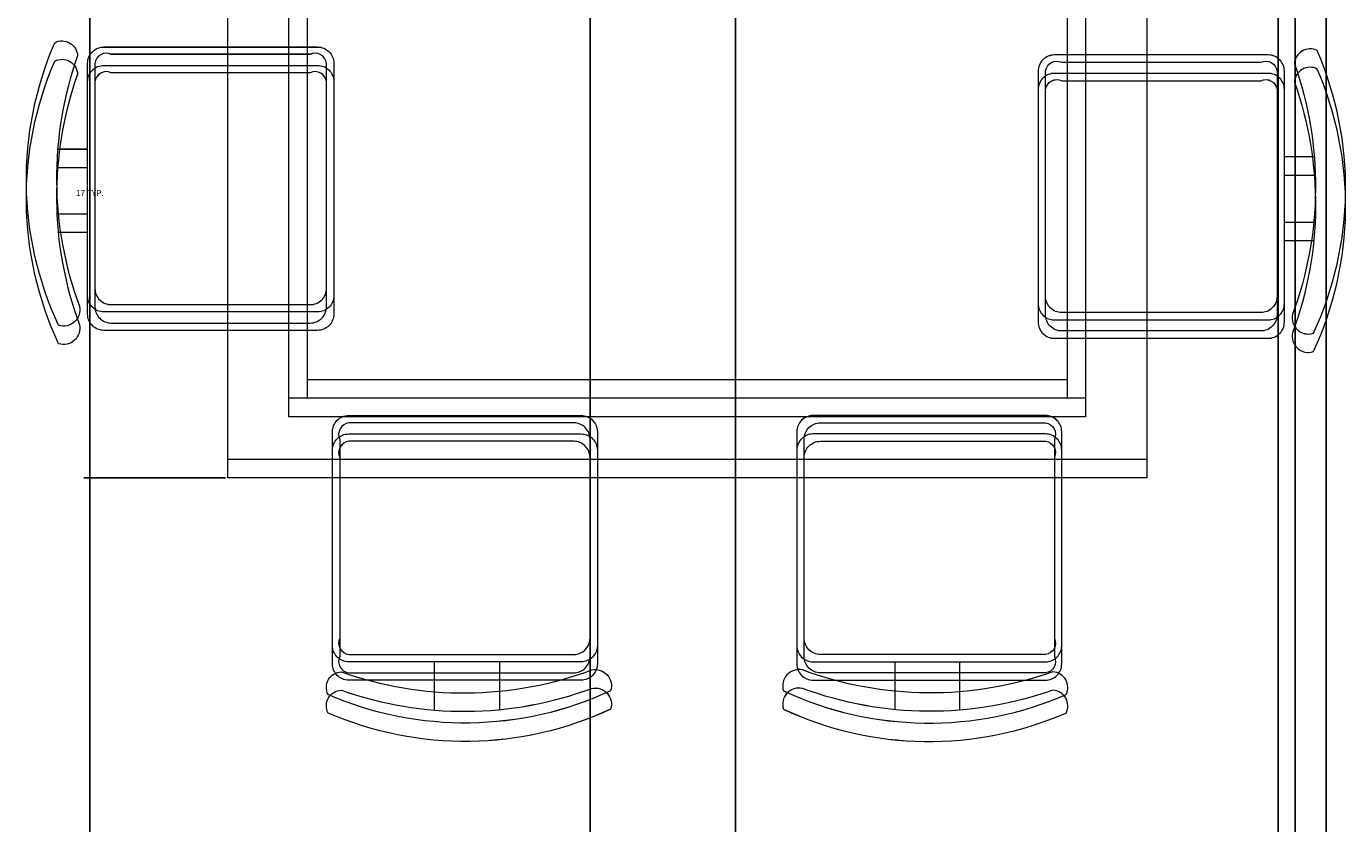
# Model space of a CAD drawing. Units: inches. Extents: x 2063 to 2617, y 1299 to 2210.
# Tile 10 of 22: x 2243 to 2282, y 1901 to 1925. Entities that reach past the tile are written whole.
import ezdxf

# ---------------------------------------------------------------- set-up
doc = ezdxf.new("R2010")
doc.units = ezdxf.units.IN
doc.layers.add('A-ANNO-DIMS', color=2, linetype='Continuous', lineweight=18)
doc.layers.add('A-FURN', color=8, linetype='Continuous', lineweight=18)
doc.styles.get("Standard").update_dxf_attribs({"font": 'arial.ttf'})
doc.dimstyles.get("Standard").update_dxf_attribs({"dimtxt": 0.18, "dimasz": 0.18, "dimexe": 0.18, "dimexo": 0.0625, "dimgap": 0.09, "dimtad": 0, "dimtih": 1, "dimtoh": 1, "dimdec": 4, "dimzin": 0, "dimdsep": 46, "dimtxsty": 'Standard', "dimcen": 0.09, "dimadec": 0, "dimazin": 0, "dimtfac": 1, "dimtdec": 4, "dimtofl": 0, "dimtmove": 0, "dimatfit": 3, "dimfxl": 1, "dimtolj": 1, "dimtzin": 0, "dimarcsym": 0})

# ---------------------------------------------------------------- blocks, each defined once
blk = doc.blocks.new('TABLE-DINING')
for points in [[(0, 17.017), (27.446, 17.017), (27.446, 0.549), (0, 0.549)], [(0, 17.017), (27.446, 17.017), (27.446, 0.549), (0, 0.549)], [(0, 17.016), (27.446, 17.016), (27.446, 0.549), (0, 0.549)], [(0, 17.016), (27.446, 17.016), (27.446, 0.549), (0, 0.549)], [(0, 16.468), (27.446, 16.468), (27.446, 0), (0, 0)], [(0, 16.468), (27.446, 16.468), (27.446, 0), (0, 0)], [(0, 16.467), (27.446, 16.467), (27.446, 0), (0, 0)], [(0, 16.467), (27.446, 16.467), (27.446, 0), (0, 0)], [(1.83, 15.187), (25.616, 15.187), (25.616, 2.379), (1.83, 2.379)], [(1.83, 15.187), (25.616, 15.187), (25.616, 2.379), (1.83, 2.379)], [(1.83, 15.187), (25.616, 15.187), (25.616, 2.379), (1.83, 2.379)], [(1.83, 15.187), (25.616, 15.187), (25.616, 2.379), (1.83, 2.379)], [(1.83, 14.638), (25.616, 14.638), (25.616, 1.83), (1.83, 1.83)], [(1.83, 14.638), (25.616, 14.638), (25.616, 1.83), (1.83, 1.83)], [(1.83, 14.638), (25.616, 14.638), (25.616, 1.83), (1.83, 1.83)], [(1.83, 14.638), (25.616, 14.638), (25.616, 1.83), (1.83, 1.83)], [(2.379, 14.638), (25.067, 14.638), (25.067, 2.928), (2.379, 2.928)], [(2.379, 14.638), (25.067, 14.638), (25.067, 2.927), (2.379, 2.927)], [(2.379, 14.638), (25.067, 14.638), (25.067, 2.928), (2.379, 2.928)], [(2.379, 14.638), (25.067, 14.638), (25.067, 2.927), (2.379, 2.927)], [(2.379, 14.089), (25.067, 14.089), (25.067, 2.379), (2.379, 2.379)], [(2.379, 14.089), (25.067, 14.089), (25.067, 2.379), (2.379, 2.379)], [(2.379, 14.089), (25.067, 14.089), (25.067, 2.379), (2.379, 2.379)], [(2.379, 14.089), (25.067, 14.089), (25.067, 2.379), (2.379, 2.379)]]:
    blk.add_lwpolyline(points, close=True)
blk = doc.blocks.new('*D26')
at = {"layer": 'A-ANNO-DIMS', "color": 0, "lineweight": -2, "transparency": 16777216}
for p, q in [((2248.921, 1928.735), (2244.686, 1928.735)), ((2244.866, 1928.555), (2244.866, 1920.407)), ((2244.866, 1911.898), (2244.866, 1920.046)), ((2248.921, 1911.718), (2244.686, 1911.718))]:
    blk.add_line(p, q, dxfattribs=at)
at = {"layer": 'A-ANNO-DIMS', "color": 0, "transparency": 16777216}
for points in [[(2244.836, 1928.555), (2244.896, 1928.555), (2244.866, 1928.735)], [(2244.836, 1911.898), (2244.896, 1911.898), (2244.866, 1911.718)]]:
    blk.add_solid(points, dxfattribs=at)
at = {"layer": 'Defpoints', "color": 0, "transparency": 16777216}
for p in [(2244.866, 1928.735), (2248.983, 1928.735), (2248.983, 1911.718)]:
    blk.add_point(p, dxfattribs=at)
at = {"layer": 'A-ANNO-DIMS', "color": 0, "transparency": 16777216, "insert": (2244.866, 1920.226), "char_height": 0.18, "attachment_point": 5}
blk.add_mtext('\\A1;17 TYP.', dxfattribs=at)
blk = doc.blocks.new('*D50')
at = {"layer": 'A-ANNO-DIMS', "color": 0, "lineweight": -2, "transparency": 16777216}
for p, q in [((2264.144, 2124.25), (2264.144, 1317.702)), ((2280.348, 2124.25), (2280.348, 1317.702)), ((2264.324, 1317.882), (2271.791, 1317.882)), ((2280.168, 1317.882), (2272.701, 1317.882))]:
    blk.add_line(p, q, dxfattribs=at)
at = {"layer": 'A-ANNO-DIMS', "color": 0, "transparency": 16777216}
for points in [[(2264.324, 1317.912), (2264.324, 1317.852), (2264.144, 1317.882)], [(2280.168, 1317.912), (2280.168, 1317.852), (2280.348, 1317.882)]]:
    blk.add_solid(points, dxfattribs=at)
at = {"layer": 'Defpoints', "color": 0, "transparency": 16777216}
for p in [(2264.144, 2124.312), (2280.348, 2124.312), (2280.348, 1317.882)]:
    blk.add_point(p, dxfattribs=at)
at = {"layer": 'A-ANNO-DIMS', "color": 0, "transparency": 16777216, "insert": (2272.246, 1317.882), "char_height": 0.18, "attachment_point": 5}
blk.add_mtext('\\A1;16.204', dxfattribs=at)
blk = doc.blocks.new('*D62')
at = {"layer": 'A-ANNO-DIMS', "color": 0, "lineweight": -2, "transparency": 16777216}
for p, q in [((2259.809, 1437.875), (2259.809, 2170.742)), ((2281.788, 1437.875), (2281.788, 2170.742)), ((2259.989, 2170.562), (2270.403, 2170.562)), ((2281.608, 2170.562), (2271.194, 2170.562))]:
    blk.add_line(p, q, dxfattribs=at)
at = {"layer": 'A-ANNO-DIMS', "color": 0, "transparency": 16777216}
for points in [[(2259.989, 2170.592), (2259.989, 2170.532), (2259.809, 2170.562)], [(2281.608, 2170.592), (2281.608, 2170.532), (2281.788, 2170.562)]]:
    blk.add_solid(points, dxfattribs=at)
at = {"layer": 'Defpoints', "color": 0, "transparency": 16777216}
for p in [(2281.788, 2170.562), (2259.809, 1437.812), (2281.788, 1437.812)]:
    blk.add_point(p, dxfattribs=at)
at = {"layer": 'A-ANNO-DIMS', "color": 0, "transparency": 16777216, "insert": (2270.798, 2170.562), "char_height": 0.18, "attachment_point": 5}
blk.add_mtext('\\A1;21.98', dxfattribs=at)
blk = doc.blocks.new('*D63')
at = {"layer": 'A-ANNO-DIMS', "color": 0, "lineweight": -2, "transparency": 16777216}
for p, q in [((2244.867, 1562.375), (2244.867, 2170.742)), ((2280.862, 1562.375), (2280.862, 2170.742)), ((2245.047, 2170.562), (2262.4, 2170.562)), ((2280.682, 2170.562), (2263.329, 2170.562))]:
    blk.add_line(p, q, dxfattribs=at)
at = {"layer": 'A-ANNO-DIMS', "color": 0, "transparency": 16777216}
for points in [[(2245.047, 2170.592), (2245.047, 2170.532), (2244.867, 2170.562)], [(2280.682, 2170.592), (2280.682, 2170.532), (2280.862, 2170.562)]]:
    blk.add_solid(points, dxfattribs=at)
at = {"layer": 'Defpoints', "color": 0, "transparency": 16777216}
for p in [(2280.862, 2170.562), (2244.867, 1562.312), (2280.862, 1562.312)]:
    blk.add_point(p, dxfattribs=at)
at = {"layer": 'A-ANNO-DIMS', "color": 0, "transparency": 16777216, "insert": (2262.865, 2170.562), "char_height": 0.18, "attachment_point": 5}
blk.add_mtext('\\A1;35.995', dxfattribs=at)

msp = doc.modelspace()

# ---------------------------------------------------------------- linework, layer by layer
at = {"layer": 'A-FURN'}
for points in [[(2244.5572, 1916.8435, -0.5783921), (2243.9345, 1916.2772, -0.2145244), (2243.8212, 1924.7154, -0.552014), (2244.5006, 1924.319, 0.1758094), (2244.5572, 1916.8435)], [(2244.5572, 1916.8435, -0.5783921), (2243.9345, 1916.2772, -0.2145244), (2243.8212, 1924.7154, -0.552014), (2244.5006, 1924.319, 0.1758094), (2244.5572, 1916.8435)], [(2244.5572, 1916.8433, -0.5783921), (2243.9345, 1916.2769, -0.2145244), (2243.8213, 1924.7151, -0.552014), (2244.5006, 1924.3187, 0.1758094), (2244.5572, 1916.8432)], [(2244.5572, 1916.8433, -0.5783921), (2243.9345, 1916.2769, -0.2145244), (2243.8213, 1924.7151, -0.552014), (2244.5006, 1924.3187, 0.1758094), (2244.5572, 1916.8432)], [(2244.8006, 1924.1006, -0.4142136), (2245.2861, 1924.5862), (2251.6673, 1924.5862, -0.4142136), (2252.1528, 1924.1006), (2252.1528, 1917.1607, -0.4142136), (2251.6673, 1916.6752), (2245.2861, 1916.6752, -0.4142136), (2244.8006, 1917.1607), (2244.8006, 1924.1006)], [(2244.8006, 1924.1006, -0.4142136), (2245.2861, 1924.5862), (2251.6673, 1924.5862, -0.4142136), (2252.1528, 1924.1006), (2252.1528, 1917.1607, -0.4142136), (2251.6673, 1916.6752), (2245.2861, 1916.6752, -0.4142136), (2244.8006, 1917.1607), (2244.8006, 1924.1006)], [(2244.8006, 1924.1003, -0.4142136), (2245.2861, 1924.5859), (2251.6673, 1924.5859, -0.4142136), (2252.1528, 1924.1003), (2252.1528, 1917.1604, -0.4142136), (2251.6673, 1916.6749), (2245.2861, 1916.6749, -0.4142136), (2244.8006, 1917.1604), (2244.8006, 1924.1003)], [(2244.8006, 1924.1003, -0.4142136), (2245.2861, 1924.5859), (2251.6673, 1924.5859, -0.4142136), (2252.1528, 1924.1003), (2252.1528, 1917.1604, -0.4142136), (2251.6673, 1916.6749), (2245.2861, 1916.6749, -0.4142136), (2244.8006, 1917.1604), (2244.8006, 1924.1003)], [(2280.8381, 1924.0813, -0.1758092), (2280.7815, 1916.6059, 0.5783921), (2281.4042, 1916.0395, 0.2145244), (2281.5174, 1924.4777, 0.552014), (2280.8381, 1924.0813, -0.065079)], [(2280.8381, 1924.0813, -0.1758092), (2280.7815, 1916.6059, 0.5783921), (2281.4042, 1916.0395, 0.2145244), (2281.5174, 1924.4777, 0.552014), (2280.8381, 1924.0813, -0.065079)], [(2280.8381, 1924.081, -0.1758092), (2280.7815, 1916.6056, 0.5783921), (2281.4042, 1916.0392, 0.2145244), (2281.5174, 1924.4774, 0.552014), (2280.8381, 1924.081, -0.065079)], [(2280.8381, 1924.081, -0.1758092), (2280.7815, 1916.6056, 0.5783921), (2281.4042, 1916.0392, 0.2145244), (2281.5174, 1924.4774, 0.552014), (2280.8381, 1924.081, -0.065079)], [(2244.5572, 1916.2946, -0.5783921), (2243.9345, 1915.7283, -0.2145244), (2243.8212, 1924.1665, -0.552014), (2244.5006, 1923.7701, 0.1758094), (2244.5572, 1916.2946)], [(2244.5572, 1916.2946, -0.5783921), (2243.9345, 1915.7283, -0.2145244), (2243.8212, 1924.1665, -0.552014), (2244.5006, 1923.7701, 0.1758094), (2244.5572, 1916.2946)], [(2244.5572, 1916.2943, -0.5783921), (2243.9345, 1915.728, -0.2145244), (2243.8213, 1924.1662, -0.552014), (2244.5006, 1923.7698, 0.1758094), (2244.5572, 1916.2943)], [(2244.5572, 1916.2943, -0.5783921), (2243.9345, 1915.728, -0.2145244), (2243.8213, 1924.1662, -0.552014), (2244.5006, 1923.7698, 0.1758094), (2244.5572, 1916.2943)], [(2280.5381, 1923.863, 0.4142136), (2280.0525, 1924.3485), (2273.6714, 1924.3485, 0.4142136), (2273.1859, 1923.863), (2273.1859, 1916.923, 0.4142136), (2273.6714, 1916.4375), (2280.0525, 1916.4375, 0.4142136), (2280.5381, 1916.923), (2280.5381, 1923.863)], [(2280.5381, 1923.863, 0.4142136), (2280.0525, 1924.3485), (2273.6714, 1924.3485, 0.4142136), (2273.1859, 1923.863), (2273.1859, 1916.923, 0.4142136), (2273.6714, 1916.4375), (2280.0525, 1916.4375, 0.4142136), (2280.5381, 1916.923), (2280.5381, 1923.863)], [(2280.5381, 1923.8627, 0.4142136), (2280.0526, 1924.3482), (2273.6714, 1924.3482, 0.4142136), (2273.1859, 1923.8627), (2273.1859, 1916.9227, 0.4142136), (2273.6714, 1916.4372), (2280.0526, 1916.4372, 0.4142136), (2280.5381, 1916.9227), (2280.5381, 1923.8627)], [(2280.5381, 1923.8627, 0.4142136), (2280.0526, 1924.3482), (2273.6714, 1924.3482, 0.4142136), (2273.1859, 1923.8627), (2273.1859, 1916.9227, 0.4142136), (2273.6714, 1916.4372), (2280.0526, 1916.4372, 0.4142136), (2280.5381, 1916.9227), (2280.5381, 1923.8627)], [(2244.8006, 1923.5517, -0.4142136), (2245.2861, 1924.0372), (2251.6673, 1924.0372, -0.4142136), (2252.1528, 1923.5517), (2252.1528, 1916.6118, -0.4142136), (2251.6673, 1916.1262), (2245.2861, 1916.1262, -0.4142136), (2244.8006, 1916.6118), (2244.8006, 1923.5517)], [(2244.8006, 1923.5517, -0.4142136), (2245.2861, 1924.0372), (2251.6673, 1924.0372, -0.4142136), (2252.1528, 1923.5517), (2252.1528, 1916.6118, -0.4142136), (2251.6673, 1916.1262), (2245.2861, 1916.1262, -0.4142136), (2244.8006, 1916.6118), (2244.8006, 1923.5517)], [(2244.8006, 1923.5514, -0.4142136), (2245.2861, 1924.037), (2251.6673, 1924.037, -0.4142136), (2252.1528, 1923.5514), (2252.1528, 1916.6115, -0.4142136), (2251.6673, 1916.126), (2245.2861, 1916.126, -0.4142136), (2244.8006, 1916.6115), (2244.8006, 1923.5514)], [(2244.8006, 1923.5514, -0.4142136), (2245.2861, 1924.037), (2251.6673, 1924.037, -0.4142136), (2252.1528, 1923.5514), (2252.1528, 1916.6115, -0.4142136), (2251.6673, 1916.126), (2245.2861, 1916.126, -0.4142136), (2244.8006, 1916.6115), (2244.8006, 1923.5514)], [(2280.5381, 1923.314, 0.4142136), (2280.0525, 1923.7996), (2273.6714, 1923.7996, 0.4142136), (2273.1859, 1923.314), (2273.1859, 1916.3741, 0.4142136), (2273.6714, 1915.8886), (2280.0525, 1915.8886, 0.4142136), (2280.5381, 1916.3741), (2280.5381, 1923.314)], [(2280.5381, 1923.314, 0.4142136), (2280.0525, 1923.7996), (2273.6714, 1923.7996, 0.4142136), (2273.1859, 1923.314), (2273.1859, 1916.3741, 0.4142136), (2273.6714, 1915.8886), (2280.0525, 1915.8886, 0.4142136), (2280.5381, 1916.3741), (2280.5381, 1923.314)], [(2280.5381, 1923.3138, 0.4142136), (2280.0526, 1923.7993), (2273.6714, 1923.7993, 0.4142136), (2273.1859, 1923.3138), (2273.1859, 1916.3738, 0.4142136), (2273.6714, 1915.8883), (2280.0526, 1915.8883, 0.4142136), (2280.5381, 1916.3738), (2280.5381, 1923.3138)], [(2280.5381, 1923.3138, 0.4142136), (2280.0526, 1923.7993), (2273.6714, 1923.7993, 0.4142136), (2273.1859, 1923.3138), (2273.1859, 1916.3738, 0.4142136), (2273.6714, 1915.8883), (2280.0526, 1915.8883, 0.4142136), (2280.5381, 1916.3738), (2280.5381, 1923.3138)], [(2280.8381, 1923.5324, -0.1758092), (2280.7815, 1916.0569, 0.5783921), (2281.4042, 1915.4906, 0.2145244), (2281.5174, 1923.9288, 0.552014), (2280.8381, 1923.5324, -0.065079)], [(2280.8381, 1923.5324, -0.1758092), (2280.7815, 1916.0569, 0.5783921), (2281.4042, 1915.4906, 0.2145244), (2281.5174, 1923.9288, 0.552014), (2280.8381, 1923.5324, -0.065079)], [(2280.8381, 1923.5321, -0.1758092), (2280.7815, 1916.0567, 0.5783921), (2281.4042, 1915.4903, 0.2145244), (2281.5174, 1923.9285, 0.552014), (2280.8381, 1923.5321, -0.065079)], [(2280.8381, 1923.5321, -0.1758092), (2280.7815, 1916.0567, 0.5783921), (2281.4042, 1915.4903, 0.2145244), (2281.5174, 1923.9285, 0.552014), (2280.8381, 1923.5321, -0.065079)], [(2244.8006, 1919.5983), (2243.9229, 1919.5983, 0.0647586)], [(2244.8006, 1919.5983), (2243.9229, 1919.5983, 0.0647586)], [(2244.8006, 1919.5981), (2243.9229, 1919.5981, 0.0647586)], [(2244.8006, 1919.5981), (2243.9229, 1919.5981, 0.0647586)], [(2280.5381, 1919.3607), (2281.4158, 1919.3607, -0.0647586)], [(2280.5381, 1919.3607), (2281.4158, 1919.3607, -0.0647586)], [(2280.5381, 1919.3604), (2281.4158, 1919.3604, -0.0647586)], [(2280.5381, 1919.3604), (2281.4158, 1919.3604, -0.0647586)], [(2244.8006, 1919.0494), (2243.9229, 1919.0494, 0.0647586)], [(2244.8006, 1919.0494), (2243.9229, 1919.0494, 0.0647586)], [(2244.8006, 1919.0491), (2243.9229, 1919.0491, 0.0647586)], [(2244.8006, 1919.0491), (2243.9229, 1919.0491, 0.0647586)], [(2280.5381, 1918.8118), (2281.4158, 1918.8118, -0.0647586)], [(2280.5381, 1918.8118), (2281.4158, 1918.8118, -0.0647586)], [(2280.5381, 1918.8115), (2281.4158, 1918.8115, -0.0647586)], [(2280.5381, 1918.8115), (2281.4158, 1918.8115, -0.0647586)], [(2259.5362, 1906.2298), (2252.5963, 1906.2298, -0.4142136), (2252.1107, 1906.7153), (2252.1107, 1913.0965, -0.4142136), (2252.5963, 1913.582), (2259.5362, 1913.582, -0.4142136), (2260.0217, 1913.0965), (2260.0217, 1906.7153, -0.4142136), (2259.5362, 1906.2298)], [(2259.5362, 1906.2298), (2252.5963, 1906.2298, -0.4142136), (2252.1107, 1906.7153), (2252.1107, 1913.0965, -0.4142136), (2252.5963, 1913.582), (2259.5362, 1913.582, -0.4142136), (2260.0217, 1913.0965), (2260.0217, 1906.7153, -0.4142136), (2259.5362, 1906.2298)], [(2259.5362, 1906.2295), (2252.5963, 1906.2295, -0.4142136), (2252.1108, 1906.715), (2252.1108, 1913.0962, -0.4142136), (2252.5963, 1913.5817), (2259.5362, 1913.5817, -0.4142136), (2260.0218, 1913.0962), (2260.0218, 1906.715, -0.4142136), (2259.5362, 1906.2295)], [(2259.5362, 1906.2295), (2252.5963, 1906.2295, -0.4142136), (2252.1108, 1906.715), (2252.1108, 1913.0962, -0.4142136), (2252.5963, 1913.5817), (2259.5362, 1913.5817, -0.4142136), (2260.0218, 1913.0962), (2260.0218, 1906.715, -0.4142136), (2259.5362, 1906.2295)], [(2273.4038, 1906.2298, 0.4142136), (2273.8893, 1906.7153), (2273.8893, 1913.0965, 0.4142136), (2273.4038, 1913.582), (2266.4639, 1913.582, 0.4142136), (2265.9783, 1913.0965), (2265.9783, 1906.7153, 0.4142136), (2266.4639, 1906.2298), (2273.4038, 1906.2298)], [(2273.4038, 1906.2298, 0.4142136), (2273.8893, 1906.7153), (2273.8893, 1913.0965, 0.4142136), (2273.4038, 1913.582), (2266.4639, 1913.582, 0.4142136), (2265.9783, 1913.0965), (2265.9783, 1906.7153, 0.4142136), (2266.4639, 1906.2298), (2273.4038, 1906.2298)], [(2273.4038, 1906.2295, 0.4142136), (2273.8893, 1906.715), (2273.8893, 1913.0962, 0.4142136), (2273.4038, 1913.5817), (2266.4639, 1913.5817, 0.4142136), (2265.9784, 1913.0962), (2265.9784, 1906.715, 0.4142136), (2266.4639, 1906.2295), (2273.4038, 1906.2295)], [(2273.4038, 1906.2295, 0.4142136), (2273.8893, 1906.715), (2273.8893, 1913.0962, 0.4142136), (2273.4038, 1913.5817), (2266.4639, 1913.5817, 0.4142136), (2265.9784, 1913.0962), (2265.9784, 1906.715, 0.4142136), (2266.4639, 1906.2295), (2273.4038, 1906.2295)], [(2259.5362, 1905.6809), (2252.5963, 1905.6809, -0.4142136), (2252.1107, 1906.1664), (2252.1107, 1912.5476, -0.4142136), (2252.5963, 1913.0331), (2259.5362, 1913.0331, -0.4142136), (2260.0217, 1912.5476), (2260.0217, 1906.1664, -0.4142136), (2259.5362, 1905.6809)], [(2259.5362, 1905.6809), (2252.5963, 1905.6809, -0.4142136), (2252.1107, 1906.1664), (2252.1107, 1912.5476, -0.4142136), (2252.5963, 1913.0331), (2259.5362, 1913.0331, -0.4142136), (2260.0217, 1912.5476), (2260.0217, 1906.1664, -0.4142136), (2259.5362, 1905.6809)], [(2259.5362, 1905.6806), (2252.5963, 1905.6806, -0.4142136), (2252.1108, 1906.1661), (2252.1108, 1912.5473, -0.4142136), (2252.5963, 1913.0328), (2259.5362, 1913.0328, -0.4142136), (2260.0218, 1912.5473), (2260.0218, 1906.1661, -0.4142136), (2259.5362, 1905.6806)], [(2259.5362, 1905.6806), (2252.5963, 1905.6806, -0.4142136), (2252.1108, 1906.1661), (2252.1108, 1912.5473, -0.4142136), (2252.5963, 1913.0328), (2259.5362, 1913.0328, -0.4142136), (2260.0218, 1912.5473), (2260.0218, 1906.1661, -0.4142136), (2259.5362, 1905.6806)], [(2273.4038, 1905.6809, 0.4142136), (2273.8893, 1906.1664), (2273.8893, 1912.5476, 0.4142136), (2273.4038, 1913.0331), (2266.4639, 1913.0331, 0.4142136), (2265.9783, 1912.5476), (2265.9783, 1906.1664, 0.4142136), (2266.4639, 1905.6809), (2273.4038, 1905.6809)], [(2273.4038, 1905.6809, 0.4142136), (2273.8893, 1906.1664), (2273.8893, 1912.5476, 0.4142136), (2273.4038, 1913.0331), (2266.4639, 1913.0331, 0.4142136), (2265.9783, 1912.5476), (2265.9783, 1906.1664, 0.4142136), (2266.4639, 1905.6809), (2273.4038, 1905.6809)], [(2273.4038, 1905.6806, 0.4142136), (2273.8893, 1906.1661), (2273.8893, 1912.5473, 0.4142136), (2273.4038, 1913.0328), (2266.4639, 1913.0328, 0.4142136), (2265.9784, 1912.5473), (2265.9784, 1906.1661, 0.4142136), (2266.4639, 1905.6806), (2273.4038, 1905.6806)], [(2273.4038, 1905.6806, 0.4142136), (2273.8893, 1906.1661), (2273.8893, 1912.5473, 0.4142136), (2273.4038, 1913.0328), (2266.4639, 1913.0328, 0.4142136), (2265.9784, 1912.5473), (2265.9784, 1906.1661, 0.4142136), (2266.4639, 1905.6806), (2273.4038, 1905.6806)], [(2259.8534, 1905.9864, -0.5783921), (2260.4197, 1905.3637, -0.2145244), (2251.9815, 1905.2505, -0.552014), (2252.3779, 1905.9298, 0.1758093), (2259.8534, 1905.9864)], [(2259.8534, 1905.9864, -0.5783921), (2260.4197, 1905.3637, -0.2145244), (2251.9815, 1905.2505, -0.552014), (2252.3779, 1905.9298, 0.1758093), (2259.8534, 1905.9864)], [(2259.8534, 1905.9861, -0.5783921), (2260.4197, 1905.3634, -0.2145244), (2251.9815, 1905.2502, -0.552014), (2252.3779, 1905.9295, 0.1758093), (2259.8534, 1905.9861)], [(2259.8534, 1905.9861, -0.5783921), (2260.4197, 1905.3634, -0.2145244), (2251.9815, 1905.2502, -0.552014), (2252.3779, 1905.9295, 0.1758093), (2259.8534, 1905.9861)], [(2257.0986, 1906.2298), (2257.0986, 1905.3521, 0.0647586)], [(2257.0986, 1906.2298), (2257.0986, 1905.3521, 0.0647586)], [(2257.0986, 1906.2295), (2257.0986, 1905.3518, 0.0647586)], [(2257.0986, 1906.2295), (2257.0986, 1905.3518, 0.0647586)], [(2273.6222, 1905.9298, -0.1758093), (2266.1467, 1905.9864, 0.5783921), (2265.5804, 1905.3637, 0.2145244), (2274.0186, 1905.2505, 0.552014), (2273.6222, 1905.9298, -0.065079)], [(2273.6222, 1905.9298, -0.1758093), (2266.1467, 1905.9864, 0.5783921), (2265.5804, 1905.3637, 0.2145244), (2274.0186, 1905.2505, 0.552014), (2273.6222, 1905.9298, -0.065079)], [(2273.6222, 1905.9295, -0.1758093), (2266.1467, 1905.9861, 0.5783921), (2265.5804, 1905.3634, 0.2145244), (2274.0186, 1905.2502, 0.552014), (2273.6222, 1905.9295, -0.065079)], [(2273.6222, 1905.9295, -0.1758093), (2266.1467, 1905.9861, 0.5783921), (2265.5804, 1905.3634, 0.2145244), (2274.0186, 1905.2502, 0.552014), (2273.6222, 1905.9295, -0.065079)], [(2268.9015, 1906.2298), (2268.9015, 1905.3521, -0.0647586)], [(2268.9015, 1906.2298), (2268.9015, 1905.3521, -0.0647586)], [(2268.9015, 1906.2295), (2268.9015, 1905.3518, -0.0647586)], [(2268.9015, 1906.2295), (2268.9015, 1905.3518, -0.0647586)], [(2257.0986, 1905.6809), (2257.0986, 1904.8032, 0.0647586)], [(2257.0986, 1905.6809), (2257.0986, 1904.8032, 0.0647586)], [(2257.0986, 1905.6806), (2257.0986, 1904.8029, 0.0647586)], [(2257.0986, 1905.6806), (2257.0986, 1904.8029, 0.0647586)], [(2268.9015, 1905.6809), (2268.9015, 1904.8032, -0.0647586)], [(2268.9015, 1905.6809), (2268.9015, 1904.8032, -0.0647586)], [(2268.9015, 1905.6806), (2268.9015, 1904.8029, -0.0647586)], [(2268.9015, 1905.6806), (2268.9015, 1904.8029, -0.0647586)], [(2259.8534, 1905.4375, -0.5783921), (2260.4197, 1904.8148, -0.2145244), (2251.9815, 1904.7015, -0.552014), (2252.3779, 1905.3809, 0.1758093), (2259.8534, 1905.4375)], [(2259.8534, 1905.4375, -0.5783921), (2260.4197, 1904.8148, -0.2145244), (2251.9815, 1904.7015, -0.552014), (2252.3779, 1905.3809, 0.1758093), (2259.8534, 1905.4375)], [(2259.8534, 1905.4372, -0.5783921), (2260.4197, 1904.8145, -0.2145244), (2251.9815, 1904.7012, -0.552014), (2252.3779, 1905.3806, 0.1758093), (2259.8534, 1905.4372)], [(2259.8534, 1905.4372, -0.5783921), (2260.4197, 1904.8145, -0.2145244), (2251.9815, 1904.7012, -0.552014), (2252.3779, 1905.3806, 0.1758093), (2259.8534, 1905.4372)], [(2273.6222, 1905.3809, -0.1758093), (2266.1467, 1905.4375, 0.5783921), (2265.5804, 1904.8148, 0.2145244), (2274.0186, 1904.7015, 0.552014), (2273.6222, 1905.3809, -0.065079)], [(2273.6222, 1905.3809, -0.1758093), (2266.1467, 1905.4375, 0.5783921), (2265.5804, 1904.8148, 0.2145244), (2274.0186, 1904.7015, 0.552014), (2273.6222, 1905.3809, -0.065079)], [(2273.6222, 1905.3806, -0.1758093), (2266.1467, 1905.4372, 0.5783921), (2265.5804, 1904.8145, 0.2145244), (2274.0186, 1904.7012, 0.552014), (2273.6222, 1905.3806, -0.065079)], [(2273.6222, 1905.3806, -0.1758093), (2266.1467, 1905.4372, 0.5783921), (2265.5804, 1904.8145, 0.2145244), (2274.0186, 1904.7012, 0.552014), (2273.6222, 1905.3806, -0.065079)]]:
    msp.add_lwpolyline(points, format="xyb", dxfattribs=at)
for points in [[(2245.0193, 1924.0977), (2245.0193, 1917.3794, 0.4142136), (2245.5049, 1916.8939), (2251.4485, 1916.8939, 0.4142136), (2251.9341, 1917.3794), (2251.9341, 1924.0977, 0.5120695), (2251.4485, 1924.3674), (2245.5049, 1924.3674, 0.5120695)], [(2245.0193, 1924.0977), (2245.0193, 1917.3794, 0.4142136), (2245.5049, 1916.8939), (2251.4485, 1916.8939, 0.4142136), (2251.9341, 1917.3794), (2251.9341, 1924.0977, 0.5120695), (2251.4485, 1924.3674), (2245.5049, 1924.3674, 0.5120695)], [(2245.0193, 1924.0974), (2245.0193, 1917.3791, 0.4142136), (2245.5049, 1916.8936), (2251.4486, 1916.8936, 0.4142136), (2251.9341, 1917.3791), (2251.9341, 1924.0974, 0.5120695), (2251.4486, 1924.3671), (2245.5049, 1924.3671, 0.5120695)], [(2245.0193, 1924.0974), (2245.0193, 1917.3791, 0.4142136), (2245.5049, 1916.8936), (2251.4486, 1916.8936, 0.4142136), (2251.9341, 1917.3791), (2251.9341, 1924.0974, 0.5120695), (2251.4486, 1924.3671), (2245.5049, 1924.3671, 0.5120695)], [(2280.3193, 1923.86), (2280.3193, 1917.1417, -0.4142136), (2279.8338, 1916.6562), (2273.8901, 1916.6562, -0.4142136), (2273.4046, 1917.1417), (2273.4046, 1923.86, -0.5120695), (2273.8901, 1924.1297), (2279.8338, 1924.1297, -0.5120695)], [(2280.3193, 1923.86), (2280.3193, 1917.1417, -0.4142136), (2279.8338, 1916.6562), (2273.8901, 1916.6562, -0.4142136), (2273.4046, 1917.1417), (2273.4046, 1923.86, -0.5120695), (2273.8901, 1924.1297), (2279.8338, 1924.1297, -0.5120695)], [(2280.3193, 1923.8597), (2280.3193, 1917.1415, -0.4142136), (2279.8338, 1916.6559), (2273.8901, 1916.6559, -0.4142136), (2273.4046, 1917.1415), (2273.4046, 1923.8597, -0.5120695), (2273.8901, 1924.1295), (2279.8338, 1924.1295, -0.5120695)], [(2280.3193, 1923.8597), (2280.3193, 1917.1415, -0.4142136), (2279.8338, 1916.6559), (2273.8901, 1916.6559, -0.4142136), (2273.4046, 1917.1415), (2273.4046, 1923.8597, -0.5120695), (2273.8901, 1924.1295), (2279.8338, 1924.1295, -0.5120695)], [(2245.0193, 1923.5488), (2245.0193, 1916.8305, 0.4142136), (2245.5049, 1916.345), (2251.4485, 1916.345, 0.4142136), (2251.9341, 1916.8305), (2251.9341, 1923.5488, 0.5120695), (2251.4485, 1923.8185), (2245.5049, 1923.8185, 0.5120695)], [(2245.0193, 1923.5488), (2245.0193, 1916.8305, 0.4142136), (2245.5049, 1916.345), (2251.4485, 1916.345, 0.4142136), (2251.9341, 1916.8305), (2251.9341, 1923.5488, 0.5120695), (2251.4485, 1923.8185), (2245.5049, 1923.8185, 0.5120695)], [(2245.0193, 1923.5485), (2245.0193, 1916.8302, 0.4142136), (2245.5049, 1916.3447), (2251.4486, 1916.3447, 0.4142136), (2251.9341, 1916.8302), (2251.9341, 1923.5485, 0.5120695), (2251.4486, 1923.8182), (2245.5049, 1923.8182, 0.5120695)], [(2245.0193, 1923.5485), (2245.0193, 1916.8302, 0.4142136), (2245.5049, 1916.3447), (2251.4486, 1916.3447, 0.4142136), (2251.9341, 1916.8302), (2251.9341, 1923.5485, 0.5120695), (2251.4486, 1923.8182), (2245.5049, 1923.8182, 0.5120695)], [(2280.3193, 1923.3111), (2280.3193, 1916.5928, -0.4142136), (2279.8338, 1916.1073), (2273.8901, 1916.1073, -0.4142136), (2273.4046, 1916.5928), (2273.4046, 1923.3111, -0.5120695), (2273.8901, 1923.5808), (2279.8338, 1923.5808, -0.5120695)], [(2280.3193, 1923.3111), (2280.3193, 1916.5928, -0.4142136), (2279.8338, 1916.1073), (2273.8901, 1916.1073, -0.4142136), (2273.4046, 1916.5928), (2273.4046, 1923.3111, -0.5120695), (2273.8901, 1923.5808), (2279.8338, 1923.5808, -0.5120695)], [(2280.3193, 1923.3108), (2280.3193, 1916.5925, -0.4142136), (2279.8338, 1916.107), (2273.8901, 1916.107, -0.4142136), (2273.4046, 1916.5925), (2273.4046, 1923.3108, -0.5120695), (2273.8901, 1923.5805), (2279.8338, 1923.5805, -0.5120695)], [(2280.3193, 1923.3108), (2280.3193, 1916.5925, -0.4142136), (2279.8338, 1916.107), (2273.8901, 1916.107, -0.4142136), (2273.4046, 1916.5925), (2273.4046, 1923.3108, -0.5120695), (2273.8901, 1923.5805), (2279.8338, 1923.5805, -0.5120695)], [(2252.5992, 1906.4485), (2259.3175, 1906.4485, 0.4142136), (2259.803, 1906.9341), (2259.803, 1912.8777, 0.4142136), (2259.3175, 1913.3633), (2252.5992, 1913.3633, 0.5120695), (2252.3295, 1912.8777), (2252.3295, 1906.9341, 0.5120695)], [(2252.5992, 1906.4485), (2259.3175, 1906.4485, 0.4142136), (2259.803, 1906.9341), (2259.803, 1912.8777, 0.4142136), (2259.3175, 1913.3633), (2252.5992, 1913.3633, 0.5120695), (2252.3295, 1912.8777), (2252.3295, 1906.9341, 0.5120695)], [(2252.5992, 1906.4483), (2259.3175, 1906.4483, 0.4142136), (2259.803, 1906.9338), (2259.803, 1912.8775, 0.4142136), (2259.3175, 1913.363), (2252.5992, 1913.363, 0.5120695), (2252.3295, 1912.8775), (2252.3295, 1906.9338, 0.5120695)], [(2252.5992, 1906.4483), (2259.3175, 1906.4483, 0.4142136), (2259.803, 1906.9338), (2259.803, 1912.8775, 0.4142136), (2259.3175, 1913.363), (2252.5992, 1913.363, 0.5120695), (2252.3295, 1912.8775), (2252.3295, 1906.9338, 0.5120695)], [(2273.4009, 1906.4485), (2266.6826, 1906.4485, -0.4142136), (2266.1971, 1906.9341), (2266.1971, 1912.8777, -0.4142136), (2266.6826, 1913.3633), (2273.4009, 1913.3633, -0.5120695), (2273.6706, 1912.8777), (2273.6706, 1906.9341, -0.5120695)], [(2273.4009, 1906.4485), (2266.6826, 1906.4485, -0.4142136), (2266.1971, 1906.9341), (2266.1971, 1912.8777, -0.4142136), (2266.6826, 1913.3633), (2273.4009, 1913.3633, -0.5120695), (2273.6706, 1912.8777), (2273.6706, 1906.9341, -0.5120695)], [(2273.4009, 1906.4483), (2266.6826, 1906.4483, -0.4142136), (2266.1971, 1906.9338), (2266.1971, 1912.8775, -0.4142136), (2266.6826, 1913.363), (2273.4009, 1913.363, -0.5120695), (2273.6706, 1912.8775), (2273.6706, 1906.9338, -0.5120695)], [(2273.4009, 1906.4483), (2266.6826, 1906.4483, -0.4142136), (2266.1971, 1906.9338), (2266.1971, 1912.8775, -0.4142136), (2266.6826, 1913.363), (2273.4009, 1913.363, -0.5120695), (2273.6706, 1912.8775), (2273.6706, 1906.9338, -0.5120695)], [(2252.5992, 1905.8996), (2259.3175, 1905.8996, 0.4142136), (2259.803, 1906.3852), (2259.803, 1912.3288, 0.4142136), (2259.3175, 1912.8144), (2252.5992, 1912.8144, 0.5120695), (2252.3295, 1912.3288), (2252.3295, 1906.3852, 0.5120695)], [(2252.5992, 1905.8996), (2259.3175, 1905.8996, 0.4142136), (2259.803, 1906.3852), (2259.803, 1912.3288, 0.4142136), (2259.3175, 1912.8144), (2252.5992, 1912.8144, 0.5120695), (2252.3295, 1912.3288), (2252.3295, 1906.3852, 0.5120695)], [(2252.5992, 1905.8993), (2259.3175, 1905.8993, 0.4142136), (2259.803, 1906.3849), (2259.803, 1912.3285, 0.4142136), (2259.3175, 1912.8141), (2252.5992, 1912.8141, 0.5120695), (2252.3295, 1912.3285), (2252.3295, 1906.3849, 0.5120695)], [(2252.5992, 1905.8993), (2259.3175, 1905.8993, 0.4142136), (2259.803, 1906.3849), (2259.803, 1912.3285, 0.4142136), (2259.3175, 1912.8141), (2252.5992, 1912.8141, 0.5120695), (2252.3295, 1912.3285), (2252.3295, 1906.3849, 0.5120695)], [(2273.4009, 1905.8996), (2266.6826, 1905.8996, -0.4142136), (2266.1971, 1906.3852), (2266.1971, 1912.3288, -0.4142136), (2266.6826, 1912.8144), (2273.4009, 1912.8144, -0.5120695), (2273.6706, 1912.3288), (2273.6706, 1906.3852, -0.5120695)], [(2273.4009, 1905.8996), (2266.6826, 1905.8996, -0.4142136), (2266.1971, 1906.3852), (2266.1971, 1912.3288, -0.4142136), (2266.6826, 1912.8144), (2273.4009, 1912.8144, -0.5120695), (2273.6706, 1912.3288), (2273.6706, 1906.3852, -0.5120695)], [(2273.4009, 1905.8993), (2266.6826, 1905.8993, -0.4142136), (2266.1971, 1906.3849), (2266.1971, 1912.3285, -0.4142136), (2266.6826, 1912.8141), (2273.4009, 1912.8141, -0.5120695), (2273.6706, 1912.3285), (2273.6706, 1906.3849, -0.5120695)], [(2273.4009, 1905.8993), (2266.6826, 1905.8993, -0.4142136), (2266.1971, 1906.3849), (2266.1971, 1912.3285, -0.4142136), (2266.6826, 1912.8141), (2273.4009, 1912.8141, -0.5120695), (2273.6706, 1912.3285), (2273.6706, 1906.3849, -0.5120695)]]:
    msp.add_lwpolyline(points, format="xyb", close=True, dxfattribs=at)
for points in [[(2243.907, 1921.5409), (2244.8006, 1921.5409)], [(2243.907, 1921.5409), (2244.8006, 1921.5409)], [(2243.907, 1921.5407), (2244.8006, 1921.5407)], [(2243.907, 1921.5407), (2244.8006, 1921.5407)], [(2281.4317, 1921.3033), (2280.5381, 1921.3033)], [(2281.4317, 1921.3033), (2280.5381, 1921.3033)], [(2281.4317, 1921.303), (2280.5381, 1921.303)], [(2281.4317, 1921.303), (2280.5381, 1921.303)], [(2243.907, 1920.992), (2244.8006, 1920.992)], [(2243.907, 1920.992), (2244.8006, 1920.992)], [(2243.907, 1920.9917), (2244.8006, 1920.9917)], [(2243.907, 1920.9917), (2244.8006, 1920.9917)], [(2281.4317, 1920.7543), (2280.5381, 1920.7543)], [(2281.4317, 1920.7543), (2280.5381, 1920.7543)], [(2281.4317, 1920.7541), (2280.5381, 1920.7541)], [(2281.4317, 1920.7541), (2280.5381, 1920.7541)], [(2255.156, 1905.3362), (2255.156, 1906.2298)], [(2255.156, 1905.3362), (2255.156, 1906.2298)], [(2255.156, 1905.3359), (2255.156, 1906.2295)], [(2255.156, 1905.3359), (2255.156, 1906.2295)], [(2270.8441, 1905.3362), (2270.8441, 1906.2298)], [(2270.8441, 1905.3362), (2270.8441, 1906.2298)], [(2270.8441, 1905.3359), (2270.8441, 1906.2295)], [(2270.8441, 1905.3359), (2270.8441, 1906.2295)], [(2255.156, 1904.7873), (2255.156, 1905.6809)], [(2255.156, 1904.7873), (2255.156, 1905.6809)], [(2255.156, 1904.787), (2255.156, 1905.6806)], [(2255.156, 1904.787), (2255.156, 1905.6806)], [(2270.8441, 1904.7873), (2270.8441, 1905.6809)], [(2270.8441, 1904.7873), (2270.8441, 1905.6809)], [(2270.8441, 1904.787), (2270.8441, 1905.6806)], [(2270.8441, 1904.787), (2270.8441, 1905.6806)]]:
    msp.add_lwpolyline(points, dxfattribs=at)

# ---------------------------------------------------------------- block references
msp.add_blockref('TABLE-DINING', (2248.983, 1911.718), dxfattribs=at)

# ---------------------------------------------------------------- dimensions: what is measured, and where the dimension line sits
at = {"layer": 'A-ANNO-DIMS'}
for base, p1, p2, override, picture, middle in [((2280.8619, 2170.5622), (2244.8673, 1562.3122), (2280.8619, 1562.3122), {"dimdec": 3, "dimlfac": 1, "dimrnd": 0, "dimzin": 0, "dimdsep": 46, "dimlunit": 2}, '*D63', (2262.8646, 2170.5622)), ((2281.7879, 2170.5622), (2259.809, 1437.8122), (2281.7879, 1437.8122), {"dimdec": 2, "dimlfac": 1, "dimrnd": 0, "dimzin": 0, "dimdsep": 46, "dimlunit": 2}, '*D62', (2270.7984, 2170.5622)), ((2280.3482, 1317.8821), (2264.1442, 2124.3122), (2280.3482, 2124.3122), {"dimdec": 3, "dimlfac": 1, "dimrnd": 0, "dimzin": 0, "dimdsep": 46, "dimlunit": 2}, '*D50', (2272.2462, 1317.8821))]:
    dim = msp.add_linear_dim(base=base, p1=p1, p2=p2, dimstyle='Standard', override=override, dxfattribs=at)
    dim.commit()
    dim.dimension.update_dxf_attribs({"geometry": picture, "text_midpoint": middle})
dim = msp.add_linear_dim(base=(2244.8663, 1928.7346), p1=(2248.9832, 1911.718), p2=(2248.9832, 1928.7346), angle=90, text='<> TYP.', dimstyle='Standard', override={"dimdec": 0, "dimlfac": 1, "dimrnd": 0, "dimzin": 0, "dimdsep": 46, "dimlunit": 2}, dxfattribs=at)
dim.commit()
dim.dimension.update_dxf_attribs({"geometry": '*D26', "text_midpoint": (2244.8663, 1920.2263)})

doc.saveas('drawing.dxf')
